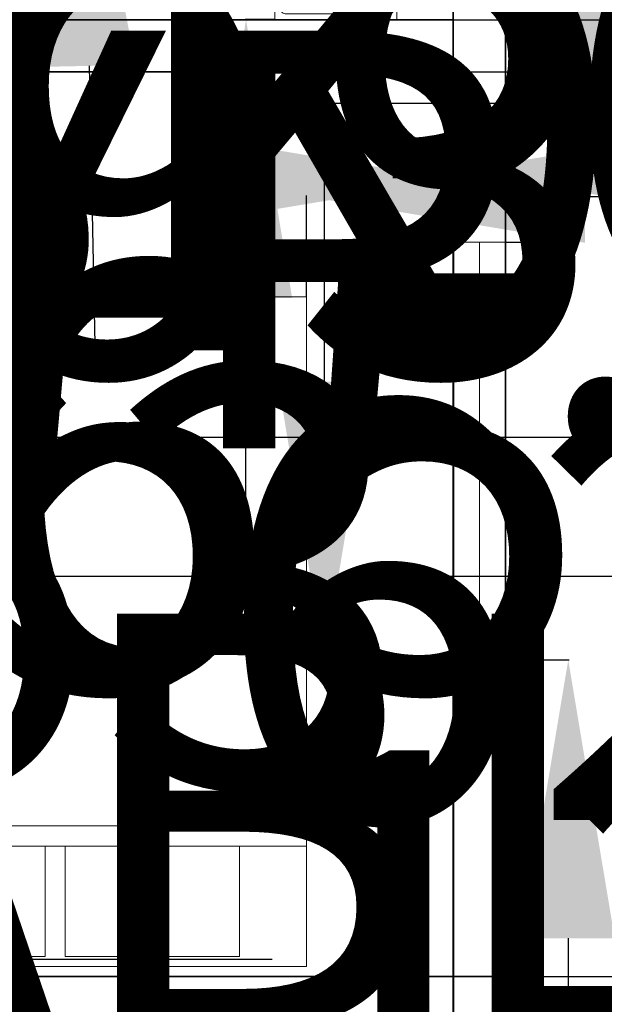
# Model space of a CAD drawing. Units: inches. Extents: x -307 to 2141, y -58 to 895.
# Tile 16 of 28: x 833 to 933, y 312 to 481. Entities that reach past the tile are written whole.
import ezdxf

# ---------------------------------------------------------------- set-up
doc = ezdxf.new("R2010")
doc.units = ezdxf.units.IN
doc.header["$MEASUREMENT"] = 0
for name, color, linetype, lineweight in [('A-ANNO-DIMS', 2, 'Continuous', 18), ('A-FLOR-FIXT', 9, 'Continuous', 18), ('A-FURN', 8, 'Continuous', 18), ('A-GLAZ', 4, 'Continuous', 18), ('A-WALL', 7, 'Continuous', 35)]:
    doc.layers.add(name, color=color, linetype=linetype, lineweight=lineweight)
doc.styles.get("Standard").update_dxf_attribs({"font": 'arial.ttf'})
doc.dimstyles.get("Standard").update_dxf_attribs({"dimtxt": 72, "dimasz": 48, "dimexe": 0.18, "dimexo": 0.0625, "dimgap": 0.09, "dimtad": 0, "dimtih": 1, "dimtoh": 1, "dimdec": 0, "dimrnd": 48, "dimzin": 0, "dimdsep": 46, "dimlunit": 3, "dimtxsty": 'Standard', "dimcen": 0.09, "dimadec": 0, "dimazin": 0, "dimtfac": 1, "dimtdec": 0, "dimtofl": 0, "dimtmove": 0, "dimatfit": 3, "dimfxl": 1, "dimtolj": 1, "dimtzin": 0, "dimarcsym": 0})

# ---------------------------------------------------------------- blocks, each defined once
blk = doc.blocks.new('Bed - Queen')
for p, q in [((0, -80.00003), (0, 0)), ((0, 0), (59.99999, 0)), ((59.99999, 0), (59.99999, -80.00003)), ((7.99999, -1.2), (28.79998, -1.2)), ((7.99999, -14.4), (7.99999, -1.2)), ((28.79998, -1.2), (28.79998, -14.4)), ((31.19999, -1.2), (51.99999, -1.2)), ((31.19999, -14.4), (31.19999, -1.2)), ((51.99999, -1.2), (51.99999, -16.4)), ((0, -14.4), (44.8, -14.4)), ((59.99999, -29.6), (44.8, -14.4)), ((44.8, -14.4), (44.8, -29.6)), ((51.99999, -16.4), (46.79936, -16.4)), ((44.8, -16.8), (0, -16.8)), ((44.8, -29.6), (59.99999, -29.6)), ((59.99999, -80.00003), (0, -80.00003))]:
    blk.add_line(p, q)
blk = doc.blocks.new('Toilet - top')
for p, q in [((9.5, -6), (9.5, -2)), ((-8, -8.5), (-8, -8)), ((-7, -8), (-7, -9.5)), ((-4, -8), (-6, -14)), ((4, -8), (6, -14)), ((-10, -8.5), (-8, -8.5)), ((-10, -9.5), (-10, -8.5)), ((-7, -9.5), (-10, -9.5)), ((4, -14), (-4, -14))]:
    blk.add_line(p, q)
blk.add_lwpolyline([(10.5, -8), (10.5, 0), (-10.5, 0), (-10.5, -8)], close=True)
for points in [[(8.5, -1), (-8.5, -1)], [(-9.5, -2), (-9.5, -6)], [(-8.5, -7), (8.5, -7)]]:
    blk.add_lwpolyline(points)
for centre, radius, start, end in [((-8.62, -1.88), 0.884, 81.8699, 188.1301), ((8.62, -1.88), 0.884, 351.8699, 98.1301), ((-8.62, -6.12), 0.884, 171.8699, 278.1301), ((8.62, -6.12), 0.884, 261.8699, 8.1301), ((3.52, -21.58), 12.17, 141.4691, 247.9714), ((4.2, -21.82), 11.33, 136.3677, 238.9468), ((-3.52, -21.58), 12.17, 292.0284, 38.5307), ((-4.2, -21.82), 11.33, 301.053, 43.6321), ((0, -27.88), 4, 245.7318, 294.2682), ((0, -29), 4, 254.8605, 285.1395)]:
    blk.add_arc(centre, radius, start, end)
blk = doc.blocks.new('WIN-36IN-PAIR')
for p, q in [((72.02, 9), (72.02, 0)), ((0, 4.5), (36, 4.5)), ((36.02, 4.5), (72.02, 4.5))]:
    blk.add_line(p, q)
for points in [[(36, 0), (0, 0), (0, 9), (36, 9)], [(36.02, 9), (72.02, 9)], [(72.02, 0), (36.02, 0)]]:
    blk.add_lwpolyline(points)
blk = doc.blocks.new('*D29')
at = {"layer": 'A-ANNO-DIMS', "color": 0, "lineweight": -2, "transparency": 16777216}
for p, q in [((747.42, 450.87), (699.42, 450.87)), ((795.42, 433.61), (795.42, 451.05)), ((882.03, 433.61), (882.03, 451.05)), ((930.03, 450.87), (978.03, 450.87))]:
    blk.add_line(p, q, dxfattribs=at)
at = {"layer": 'A-ANNO-DIMS', "color": 0, "transparency": 16777216}
for points in [[(747.42, 458.87), (747.42, 442.87), (795.42, 450.87)], [(930.03, 458.87), (930.03, 442.87), (882.03, 450.87)]]:
    blk.add_solid(points, dxfattribs=at)
at = {"layer": 'Defpoints', "color": 0, "transparency": 16777216}
for p in [(795.42, 450.87), (795.42, 433.55), (882.03, 433.55)]:
    blk.add_point(p, dxfattribs=at)
at = {"layer": 'A-ANNO-DIMS', "color": 0, "transparency": 16777216, "insert": (647.71, 450.87), "char_height": 72, "attachment_point": 5}
blk.add_mtext('\\A1;87', dxfattribs=at)
blk = doc.blocks.new('*D30')
at = {"layer": 'A-ANNO-DIMS', "color": 0, "lineweight": -2, "transparency": 16777216}
for p, q in [((570.74, 532.83), (570.74, 580.83)), ((570.74, 580.83), (618.74, 580.83)), ((565.4, 484.83), (570.92, 484.83)), ((565.4, 448.83), (570.92, 448.83)), ((570.74, 400.83), (570.74, 352.83))]:
    blk.add_line(p, q, dxfattribs=at)
at = {"layer": 'A-ANNO-DIMS', "color": 0, "transparency": 16777216}
for points in [[(562.74, 532.83), (578.74, 532.83), (570.74, 484.83)], [(562.74, 400.83), (578.74, 400.83), (570.74, 448.83)]]:
    blk.add_solid(points, dxfattribs=at)
at = {"layer": 'Defpoints', "color": 0, "transparency": 16777216}
for p in [(565.34, 484.83), (570.74, 484.83), (565.34, 448.83)]:
    blk.add_point(p, dxfattribs=at)
at = {"layer": 'A-ANNO-DIMS', "color": 0, "transparency": 16777216, "insert": (1030.17, 580.83), "char_height": 72, "attachment_point": 5}
blk.add_mtext('\\A1;WINDOW 36 TYP.', dxfattribs=at)
blk = doc.blocks.new('*D31')
at = {"layer": 'A-ANNO-DIMS', "color": 0, "lineweight": -2, "transparency": 16777216}
for p, q in [((556.34, 448.77), (556.34, 443.25)), ((565.34, 448.77), (565.34, 443.25)), ((508.34, 443.43), (460.34, 443.43)), ((613.34, 443.43), (661.34, 443.43))]:
    blk.add_line(p, q, dxfattribs=at)
at = {"layer": 'A-ANNO-DIMS', "color": 0, "transparency": 16777216}
for points in [[(508.34, 451.43), (508.34, 435.43), (556.34, 443.43)], [(613.34, 451.43), (613.34, 435.43), (565.34, 443.43)]]:
    blk.add_solid(points, dxfattribs=at)
at = {"layer": 'Defpoints', "color": 0, "transparency": 16777216}
for p in [(556.34, 448.83), (565.34, 448.83), (565.34, 443.43)]:
    blk.add_point(p, dxfattribs=at)
at = {"layer": 'A-ANNO-DIMS', "color": 0, "transparency": 16777216, "insert": (808.69, 443.43), "char_height": 72, "attachment_point": 5}
blk.add_mtext('\\A1;9 TYP.', dxfattribs=at)
blk = doc.blocks.new('*D34')
at = {"layer": 'A-ANNO-DIMS', "color": 0, "lineweight": -2, "transparency": 16777216}
for p, q in [((927.14, 490.97), (927.14, 538.97)), ((927.14, 538.97), (975.14, 538.97)), ((916.4, 442.97), (927.32, 442.97)), ((916.4, 370.95), (927.32, 370.95)), ((927.14, 322.95), (927.14, 274.95))]:
    blk.add_line(p, q, dxfattribs=at)
at = {"layer": 'A-ANNO-DIMS', "color": 0, "transparency": 16777216}
for points in [[(919.14, 490.97), (935.14, 490.97), (927.14, 442.97)], [(919.14, 322.95), (935.14, 322.95), (927.14, 370.95)]]:
    blk.add_solid(points, dxfattribs=at)
at = {"layer": 'Defpoints', "color": 0, "transparency": 16777216}
for p in [(916.34, 442.97), (927.14, 442.97), (916.34, 370.95)]:
    blk.add_point(p, dxfattribs=at)
at = {"layer": 'A-ANNO-DIMS', "color": 0, "transparency": 16777216, "insert": (1584.53, 538.97), "char_height": 72, "attachment_point": 5}
blk.add_mtext('\\A1;PAIRED WINDOW 72 TYP.', dxfattribs=at)
blk = doc.blocks.new('*D35')
at = {"layer": 'A-ANNO-DIMS', "color": 0, "lineweight": -2, "transparency": 16777216}
for p, q in [((859.34, 453.77), (811.34, 453.77)), ((907.34, 443.03), (907.34, 453.95)), ((916.34, 443.03), (916.34, 453.95)), ((964.34, 453.77), (1012.34, 453.77))]:
    blk.add_line(p, q, dxfattribs=at)
at = {"layer": 'A-ANNO-DIMS', "color": 0, "transparency": 16777216}
for points in [[(859.34, 461.77), (859.34, 445.77), (907.34, 453.77)], [(964.34, 461.77), (964.34, 445.77), (916.34, 453.77)]]:
    blk.add_solid(points, dxfattribs=at)
at = {"layer": 'Defpoints', "color": 0, "transparency": 16777216}
for p in [(907.34, 453.77), (907.34, 442.97), (916.34, 442.97)]:
    blk.add_point(p, dxfattribs=at)
at = {"layer": 'A-ANNO-DIMS', "color": 0, "transparency": 16777216, "insert": (663.98, 453.77), "char_height": 72, "attachment_point": 5}
blk.add_mtext('\\A1;9 TYP.', dxfattribs=at)
blk = doc.blocks.new('*D36')
at = {"layer": 'A-ANNO-DIMS', "color": 0, "lineweight": -2, "transparency": 16777216}
for p, q in [((871.71, 562.4), (871.76, 610.4)), ((876.55, 514.4), (871.47, 514.4)), ((876.51, 481.35), (871.44, 481.36)), ((871.56, 433.36), (871.51, 385.36)), ((871.51, 385.36), (823.51, 385.36))]:
    blk.add_line(p, q, dxfattribs=at)
at = {"layer": 'A-ANNO-DIMS', "color": 0, "transparency": 16777216}
for points in [[(863.71, 562.41), (879.71, 562.4), (871.65, 514.4)], [(863.56, 433.37), (879.56, 433.35), (871.62, 481.36)]]:
    blk.add_solid(points, dxfattribs=at)
at = {"layer": 'Defpoints', "color": 0, "transparency": 16777216}
for p in [(876.61, 514.4), (871.62, 481.36), (876.57, 481.35)]:
    blk.add_point(p, dxfattribs=at)
at = {"layer": 'A-ANNO-DIMS', "color": 0, "transparency": 16777216, "insert": (548.95, 385.36), "char_height": 72, "attachment_point": 5}
blk.add_mtext('\\A1;WC 33 TYP.', dxfattribs=at)
blk = doc.blocks.new('*D37')
at = {"layer": 'A-ANNO-DIMS', "color": 0, "lineweight": -2, "transparency": 16777216}
for p, q in [((876.61, 514.46), (876.62, 519.54)), ((828.62, 519.41), (780.62, 519.46)), ((897.61, 514.44), (897.62, 519.51)), ((945.62, 519.28), (993.62, 519.22))]:
    blk.add_line(p, q, dxfattribs=at)
at = {"layer": 'A-ANNO-DIMS', "color": 0, "transparency": 16777216}
for points in [[(828.63, 527.41), (828.61, 511.41), (876.62, 519.36)], [(945.63, 527.28), (945.61, 511.28), (897.62, 519.33)]]:
    blk.add_solid(points, dxfattribs=at)
at = {"layer": 'Defpoints', "color": 0, "transparency": 16777216}
for p in [(876.62, 519.36), (876.61, 514.4), (897.61, 514.38)]:
    blk.add_point(p, dxfattribs=at)
at = {"layer": 'A-ANNO-DIMS', "color": 0, "transparency": 16777216, "insert": (604.68, 519.46), "char_height": 72, "attachment_point": 5}
blk.add_mtext('\\A1;21 TYP.', dxfattribs=at)
blk = doc.blocks.new('*D41')
at = {"layer": 'A-ANNO-DIMS', "color": 0, "lineweight": -2, "transparency": 16777216}
for p, q in [((768.38, 207.13), (768.38, 255.13)), ((768.38, 255.13), (816.38, 255.13)), ((762.83, 159.13), (768.56, 159.13)), ((762.83, 128.96), (768.56, 128.96)), ((768.38, 80.96), (768.38, 32.96))]:
    blk.add_line(p, q, dxfattribs=at)
at = {"layer": 'A-ANNO-DIMS', "color": 0, "transparency": 16777216}
for points in [[(760.38, 207.13), (776.38, 207.13), (768.38, 159.13)], [(760.38, 80.96), (776.38, 80.96), (768.38, 128.96)]]:
    blk.add_solid(points, dxfattribs=at)
at = {"layer": 'Defpoints', "color": 0, "transparency": 16777216}
for p in [(762.77, 159.13), (768.38, 159.13), (762.77, 128.96)]:
    blk.add_point(p, dxfattribs=at)
at = {"layer": 'A-ANNO-DIMS', "color": 0, "transparency": 16777216, "insert": (991.68, 255.13), "char_height": 72, "attachment_point": 5}
blk.add_mtext('\\A1;30 TYP.', dxfattribs=at)
blk = doc.blocks.new('*D42')
at = {"layer": 'A-ANNO-DIMS', "color": 0, "lineweight": -2, "transparency": 16777216}
for p, q in [((880.26, 543.86), (928.25, 544.87)), ((774.28, 541.63), (726.29, 540.62)), ((822.3, 541.2), (822.27, 542.82)), ((832.3, 541.41), (832.27, 543.03))]:
    blk.add_line(p, q, dxfattribs=at)
at = {"layer": 'A-ANNO-DIMS', "color": 0, "transparency": 16777216}
for points in [[(880.09, 551.86), (880.43, 535.86), (832.27, 542.85)], [(774.11, 549.63), (774.45, 533.63), (822.27, 542.64)]]:
    blk.add_solid(points, dxfattribs=at)
at = {"layer": 'Defpoints', "color": 0, "transparency": 16777216}
for p in [(832.27, 542.85), (822.3, 541.14), (832.3, 541.35)]:
    blk.add_point(p, dxfattribs=at)
at = {"layer": 'A-ANNO-DIMS', "color": 0, "transparency": 16777216, "insert": (1192.89, 544.87), "char_height": 72, "attachment_point": 5}
blk.add_mtext('\\A1;FAUCET 10', dxfattribs=at)
blk = doc.blocks.new('*D44')
at = {"layer": 'A-ANNO-DIMS', "color": 0, "lineweight": -2, "transparency": 16777216}
for p, q in [((839.87, 521.22), (839.95, 517.42)), ((815.33, 520.71), (815.41, 516.91)), ((887.94, 518.61), (935.93, 519.62)), ((767.41, 516.08), (719.42, 515.07))]:
    blk.add_line(p, q, dxfattribs=at)
at = {"layer": 'A-ANNO-DIMS', "color": 0, "transparency": 16777216}
for points in [[(887.77, 526.61), (888.11, 510.61), (839.95, 517.6)], [(767.25, 524.08), (767.58, 508.08), (815.4, 517.09)]]:
    blk.add_solid(points, dxfattribs=at)
at = {"layer": 'Defpoints', "color": 0, "transparency": 16777216}
for p in [(839.87, 521.29), (815.33, 520.77), (839.95, 517.6)]:
    blk.add_point(p, dxfattribs=at)
at = {"layer": 'A-ANNO-DIMS', "color": 0, "transparency": 16777216, "insert": (1151.16, 519.62), "char_height": 72, "attachment_point": 5}
blk.add_mtext('\\A1;BASIN 25', dxfattribs=at)
blk = doc.blocks.new('*D45')
at = {"layer": 'A-ANNO-DIMS', "color": 0, "lineweight": -2, "transparency": 16777216}
for p, q in [((841.11, 637.47), (793.11, 637.47)), ((842.12, 589.48), (841.11, 637.47)), ((839.51, 541.42), (843.31, 541.5)), ((839.93, 521.29), (843.73, 521.37)), ((844.56, 473.37), (845.57, 425.38))]:
    blk.add_line(p, q, dxfattribs=at)
at = {"layer": 'A-ANNO-DIMS', "color": 0, "transparency": 16777216}
for points in [[(850.12, 589.65), (834.12, 589.32), (843.13, 541.49)], [(852.56, 473.54), (836.56, 473.21), (843.55, 521.36)]]:
    blk.add_solid(points, dxfattribs=at)
at = {"layer": 'Defpoints', "color": 0, "transparency": 16777216}
for p in [(839.45, 541.42), (843.13, 541.49), (839.87, 521.29)]:
    blk.add_point(p, dxfattribs=at)
at = {"layer": 'A-ANNO-DIMS', "color": 0, "transparency": 16777216, "insert": (740.96, 637.47), "char_height": 72, "attachment_point": 5}
blk.add_mtext('\\A1;20', dxfattribs=at)
blk = doc.blocks.new('*D46')
at = {"layer": 'A-ANNO-DIMS', "color": 0, "lineweight": -2, "transparency": 16777216}
for p, q in [((801.41, 645.78), (801.41, 642.52)), ((822.41, 645.78), (822.41, 642.52)), ((753.41, 642.7), (705.41, 642.7)), ((870.41, 642.7), (918.41, 642.7))]:
    blk.add_line(p, q, dxfattribs=at)
at = {"layer": 'A-ANNO-DIMS', "color": 0, "transparency": 16777216}
for points in [[(753.41, 650.7), (753.41, 634.7), (801.41, 642.7)], [(870.41, 650.7), (870.41, 634.7), (822.41, 642.7)]]:
    blk.add_solid(points, dxfattribs=at)
at = {"layer": 'Defpoints', "color": 0, "transparency": 16777216}
for p in [(801.41, 645.85), (822.41, 645.85), (822.41, 642.7)]:
    blk.add_point(p, dxfattribs=at)
at = {"layer": 'A-ANNO-DIMS', "color": 0, "transparency": 16777216, "insert": (1282.7, 642.7), "char_height": 72, "attachment_point": 5}
blk.add_mtext('\\A1;DESK CHAIR 21', dxfattribs=at)
blk = doc.blocks.new('*D52')
at = {"layer": 'A-ANNO-DIMS', "color": 0, "lineweight": -2, "transparency": 16777216}
for p, q in [((660.21, 554.25), (660.21, 602.25)), ((673.8, 506.25), (660.03, 506.25)), ((673.8, 415.25), (660.03, 415.25)), ((660.21, 367.25), (660.21, 319.25))]:
    blk.add_line(p, q, dxfattribs=at)
at = {"layer": 'A-ANNO-DIMS', "color": 0, "transparency": 16777216}
for points in [[(652.21, 554.25), (668.21, 554.25), (660.21, 506.25)], [(652.21, 367.25), (668.21, 367.25), (660.21, 415.25)]]:
    blk.add_solid(points, dxfattribs=at)
at = {"layer": 'Defpoints', "color": 0, "transparency": 16777216}
for p in [(673.86, 506.25), (660.21, 415.25), (673.86, 415.25)]:
    blk.add_point(p, dxfattribs=at)
at = {"layer": 'A-ANNO-DIMS', "color": 0, "transparency": 16777216, "insert": (660.21, 460.75), "char_height": 72, "attachment_point": 5}
blk.add_mtext('\\A1;DINING SET 91', dxfattribs=at)
blk = doc.blocks.new('*D53')
at = {"layer": 'A-ANNO-DIMS', "color": 0, "lineweight": -2, "transparency": 16777216}
for p, q in [((673.86, 415.19), (673.86, 401.42)), ((728.86, 415.19), (728.86, 401.42)), ((625.86, 401.6), (577.86, 401.6)), ((776.86, 401.6), (824.86, 401.6))]:
    blk.add_line(p, q, dxfattribs=at)
at = {"layer": 'A-ANNO-DIMS', "color": 0, "transparency": 16777216}
for points in [[(625.86, 409.6), (625.86, 393.6), (673.86, 401.6)], [(776.86, 409.6), (776.86, 393.6), (728.86, 401.6)]]:
    blk.add_solid(points, dxfattribs=at)
at = {"layer": 'Defpoints', "color": 0, "transparency": 16777216}
for p in [(673.86, 415.25), (728.86, 415.25), (728.86, 401.6)]:
    blk.add_point(p, dxfattribs=at)
at = {"layer": 'A-ANNO-DIMS', "color": 0, "transparency": 16777216, "insert": (876.79, 401.6), "char_height": 72, "attachment_point": 5}
blk.add_mtext('\\A1;55', dxfattribs=at)
blk = doc.blocks.new('*D54')
at = {"layer": 'A-ANNO-DIMS', "color": 0, "lineweight": -2, "transparency": 16777216}
for p, q in [((605.34, 412.35), (605.34, 460.35)), ((605.34, 460.35), (653.34, 460.35)), ((596.4, 364.35), (605.52, 364.35)), ((596.4, 304.35), (605.52, 304.35)), ((605.34, 256.35), (605.34, 208.35))]:
    blk.add_line(p, q, dxfattribs=at)
at = {"layer": 'A-ANNO-DIMS', "color": 0, "transparency": 16777216}
for points in [[(597.34, 412.35), (613.34, 412.35), (605.34, 364.35)], [(597.34, 256.35), (613.34, 256.35), (605.34, 304.35)]]:
    blk.add_solid(points, dxfattribs=at)
at = {"layer": 'Defpoints', "color": 0, "transparency": 16777216}
for p in [(596.34, 364.35), (605.34, 364.35), (596.34, 304.35)]:
    blk.add_point(p, dxfattribs=at)
at = {"layer": 'A-ANNO-DIMS', "color": 0, "transparency": 16777216, "insert": (854, 460.35), "char_height": 72, "attachment_point": 5}
blk.add_mtext('\\A1;DESK 60', dxfattribs=at)
blk = doc.blocks.new('*D60')
at = {"layer": 'A-ANNO-DIMS', "color": 0, "lineweight": -2, "transparency": 16777216}
for p, q in [((659.86, 294.95), (659.86, 342.95)), ((659.86, 342.95), (707.86, 342.95)), ((663.34, 246.95), (659.68, 246.95)), ((663.34, 223.32), (659.68, 223.32)), ((659.86, 175.32), (659.86, 127.32))]:
    blk.add_line(p, q, dxfattribs=at)
at = {"layer": 'A-ANNO-DIMS', "color": 0, "transparency": 16777216}
for points in [[(651.86, 294.95), (667.86, 294.95), (659.86, 246.95)], [(651.86, 175.32), (667.86, 175.32), (659.86, 223.32)]]:
    blk.add_solid(points, dxfattribs=at)
at = {"layer": 'Defpoints', "color": 0, "transparency": 16777216}
for p in [(659.86, 246.95), (663.4, 246.95), (663.4, 223.32)]:
    blk.add_point(p, dxfattribs=at)
at = {"layer": 'A-ANNO-DIMS', "color": 0, "transparency": 16777216, "insert": (933.57, 342.95), "char_height": 72, "attachment_point": 5}
blk.add_mtext('\\A1;TABLE 24', dxfattribs=at)
blk = doc.blocks.new('*D63')
at = {"layer": 'A-ANNO-DIMS', "color": 0, "lineweight": -2, "transparency": 16777216}
for p, q in [((916.4, 691.34), (947.72, 691.34)), ((947.54, 643.34), (947.54, 416.19)), ((947.54, 115.34), (947.54, 342.49)), ((704.68, 67.34), (947.72, 67.34))]:
    blk.add_line(p, q, dxfattribs=at)
at = {"layer": 'A-ANNO-DIMS', "color": 0, "transparency": 16777216}
for points in [[(939.54, 643.34), (955.54, 643.34), (947.54, 691.34)], [(939.54, 115.34), (955.54, 115.34), (947.54, 67.34)]]:
    blk.add_solid(points, dxfattribs=at)
at = {"layer": 'Defpoints', "color": 0, "transparency": 16777216}
for p in [(916.34, 691.34), (704.62, 67.34), (947.54, 67.34)]:
    blk.add_point(p, dxfattribs=at)
at = {"layer": 'A-ANNO-DIMS', "color": 0, "transparency": 16777216, "insert": (947.54, 379.34), "char_height": 72, "attachment_point": 5}
blk.add_mtext('\\A1;624', dxfattribs=at)
blk = doc.blocks.new('*D81')
at = {"layer": 'A-ANNO-DIMS', "color": 0, "lineweight": -2, "transparency": 16777216}
for p, q in [((947.54, 589.34), (947.54, 637.34)), ((947.54, 637.34), (995.54, 637.34)), ((907.4, 541.34), (947.72, 541.34)), ((907.4, 481.34), (947.72, 481.34)), ((947.54, 433.34), (947.54, 385.34))]:
    blk.add_line(p, q, dxfattribs=at)
at = {"layer": 'A-ANNO-DIMS', "color": 0, "transparency": 16777216}
for points in [[(939.54, 589.34), (955.54, 589.34), (947.54, 541.34)], [(939.54, 433.34), (955.54, 433.34), (947.54, 481.34)]]:
    blk.add_solid(points, dxfattribs=at)
at = {"layer": 'Defpoints', "color": 0, "transparency": 16777216}
for p in [(907.34, 541.34), (947.54, 541.34), (907.34, 481.34)]:
    blk.add_point(p, dxfattribs=at)
at = {"layer": 'A-ANNO-DIMS', "color": 0, "transparency": 16777216, "insert": (1047.27, 637.34), "char_height": 72, "attachment_point": 5}
blk.add_mtext('\\A1;60', dxfattribs=at)
blk = doc.blocks.new('*D83')
at = {"layer": 'A-ANNO-DIMS', "color": 0, "lineweight": -2, "transparency": 16777216}
for p, q in [((947.54, 538.9), (947.54, 586.9)), ((916.4, 490.9), (947.72, 490.9)), ((907.4, 481.34), (947.72, 481.34)), ((947.54, 433.34), (947.54, 385.34)), ((947.54, 385.34), (899.54, 385.34))]:
    blk.add_line(p, q, dxfattribs=at)
at = {"layer": 'A-ANNO-DIMS', "color": 0, "transparency": 16777216}
for points in [[(939.54, 538.9), (955.54, 538.9), (947.54, 490.9)], [(939.54, 433.34), (955.54, 433.34), (947.54, 481.34)]]:
    blk.add_solid(points, dxfattribs=at)
at = {"layer": 'Defpoints', "color": 0, "transparency": 16777216}
for p in [(916.34, 490.9), (907.34, 481.34), (947.54, 481.34)]:
    blk.add_point(p, dxfattribs=at)
at = {"layer": 'A-ANNO-DIMS', "color": 0, "transparency": 16777216, "insert": (777.97, 385.34), "char_height": 72, "attachment_point": 5}
blk.add_mtext('\\A1;9.563', dxfattribs=at)
blk = doc.blocks.new('*D84')
at = {"layer": 'A-ANNO-DIMS', "color": 0, "lineweight": -2, "transparency": 16777216}
for p, q in [((763.34, 472.28), (763.34, 35.96)), ((907.34, 472.28), (907.34, 35.96)), ((811.34, 36.14), (859.34, 36.14)), ((907.34, 36.14), (955.34, 36.14))]:
    blk.add_line(p, q, dxfattribs=at)
at = {"layer": 'A-ANNO-DIMS', "color": 0, "transparency": 16777216}
for points in [[(811.34, 44.14), (811.34, 28.14), (763.34, 36.14)], [(859.34, 44.14), (859.34, 28.14), (907.34, 36.14)]]:
    blk.add_solid(points, dxfattribs=at)
at = {"layer": 'Defpoints', "color": 0, "transparency": 16777216}
for p in [(763.34, 472.34), (907.34, 472.34), (907.34, 36.14)]:
    blk.add_point(p, dxfattribs=at)
at = {"layer": 'A-ANNO-DIMS', "color": 0, "transparency": 16777216, "insert": (1031.43, 36.14), "char_height": 72, "attachment_point": 5}
blk.add_mtext('\\A1;144', dxfattribs=at)
blk = doc.blocks.new('*D85')
at = {"layer": 'A-ANNO-DIMS', "color": 0, "lineweight": -2, "transparency": 16777216}
for p, q in [((947.54, 472.34), (947.54, 520.34)), ((947.54, 520.34), (995.54, 520.34)), ((907.4, 472.34), (947.72, 472.34)), ((947.54, 364.34), (947.54, 424.34)), ((916.4, 316.34), (947.72, 316.34))]:
    blk.add_line(p, q, dxfattribs=at)
at = {"layer": 'A-ANNO-DIMS', "color": 0, "transparency": 16777216}
for points in [[(939.54, 424.34), (955.54, 424.34), (947.54, 472.34)], [(939.54, 364.34), (955.54, 364.34), (947.54, 316.34)]]:
    blk.add_solid(points, dxfattribs=at)
at = {"layer": 'Defpoints', "color": 0, "transparency": 16777216}
for p in [(907.34, 472.34), (947.54, 472.34), (916.34, 316.34)]:
    blk.add_point(p, dxfattribs=at)
at = {"layer": 'A-ANNO-DIMS', "color": 0, "transparency": 16777216, "insert": (1071.76, 520.34), "char_height": 72, "attachment_point": 5}
blk.add_mtext('\\A1;156', dxfattribs=at)
blk = doc.blocks.new('*D88')
at = {"layer": 'A-ANNO-DIMS', "color": 0, "lineweight": -2, "transparency": 16777216}
for p, q in [((517.33584, 722.544828), (469.33584, 722.544828)), ((565.33584, 295.403328), (565.33584, 722.724828)), ((754.33584, 271.403328), (754.33584, 722.724828)), ((802.33584, 722.544828), (850.33584, 722.544828))]:
    blk.add_line(p, q, dxfattribs=at)
at = {"layer": 'A-ANNO-DIMS', "color": 0, "transparency": 16777216}
for points in [[(517.33584, 730.544828), (517.33584, 714.544828), (565.33584, 722.544828)], [(802.33584, 730.544828), (802.33584, 714.544828), (754.33584, 722.544828)]]:
    blk.add_solid(points, dxfattribs=at)
at = {"layer": 'Defpoints', "color": 0, "transparency": 16777216}
for p in [(754.33584, 722.544828), (565.33584, 295.340828), (754.33584, 271.340828)]:
    blk.add_point(p, dxfattribs=at)
at = {"layer": 'A-ANNO-DIMS', "color": 0, "transparency": 16777216, "insert": (659.83584, 722.544828), "char_height": 72, "attachment_point": 5}
blk.add_mtext('\\A1;189', dxfattribs=at)
blk = doc.blocks.new('*D95')
at = {"layer": 'A-ANNO-DIMS', "color": 0, "lineweight": -2, "transparency": 16777216}
for p, q in [((947.54, 577.34), (947.54, 625.34)), ((947.54, 625.34), (995.54, 625.34)), ((629.9, 529.34), (947.72, 529.34)), ((629.9, 502.66), (947.72, 502.66)), ((947.54, 454.66), (947.54, 406.66))]:
    blk.add_line(p, q, dxfattribs=at)
at = {"layer": 'A-ANNO-DIMS', "color": 0, "transparency": 16777216}
for points in [[(939.54, 577.34), (955.54, 577.34), (947.54, 529.34)], [(939.54, 454.66), (955.54, 454.66), (947.54, 502.66)]]:
    blk.add_solid(points, dxfattribs=at)
at = {"layer": 'Defpoints', "color": 0, "transparency": 16777216}
for p in [(629.84, 529.34), (947.54, 529.34), (629.84, 502.66)]:
    blk.add_point(p, dxfattribs=at)
at = {"layer": 'A-ANNO-DIMS', "color": 0, "transparency": 16777216, "insert": (1117.8, 625.34), "char_height": 72, "attachment_point": 5}
blk.add_mtext('\\A1;26.68', dxfattribs=at)
blk = doc.blocks.new('*D97')
at = {"layer": 'A-ANNO-DIMS', "color": 0, "lineweight": -2, "transparency": 16777216}
for p, q in [((947.54, 637.34), (947.54, 685.34)), ((947.54, 685.34), (995.54, 685.34)), ((685.4, 589.34), (947.72, 589.34)), ((685.4, 538.34), (947.72, 538.34)), ((947.54, 490.34), (947.54, 442.34))]:
    blk.add_line(p, q, dxfattribs=at)
at = {"layer": 'A-ANNO-DIMS', "color": 0, "transparency": 16777216}
for points in [[(939.54, 637.34), (955.54, 637.34), (947.54, 589.34)], [(939.54, 490.34), (955.54, 490.34), (947.54, 538.34)]]:
    blk.add_solid(points, dxfattribs=at)
at = {"layer": 'Defpoints', "color": 0, "transparency": 16777216}
for p in [(685.34, 589.34), (947.54, 589.34), (685.34, 538.34)]:
    blk.add_point(p, dxfattribs=at)
at = {"layer": 'A-ANNO-DIMS', "color": 0, "transparency": 16777216, "insert": (1040.25, 685.34), "char_height": 72, "attachment_point": 5}
blk.add_mtext('\\A1;51', dxfattribs=at)
blk = doc.blocks.new('*D99')
at = {"layer": 'A-ANNO-DIMS', "color": 0, "lineweight": -2, "transparency": 16777216}
for p, q in [((763.34, 481.28), (763.34, 35.96)), ((802.34, 481.28), (802.34, 35.96)), ((715.34, 36.14), (667.34, 36.14)), ((850.34, 36.14), (898.34, 36.14))]:
    blk.add_line(p, q, dxfattribs=at)
at = {"layer": 'A-ANNO-DIMS', "color": 0, "transparency": 16777216}
for points in [[(715.34, 44.14), (715.34, 28.14), (763.34, 36.14)], [(850.34, 44.14), (850.34, 28.14), (802.34, 36.14)]]:
    blk.add_solid(points, dxfattribs=at)
at = {"layer": 'Defpoints', "color": 0, "transparency": 16777216}
for p in [(763.34, 481.34), (802.34, 481.34), (802.34, 36.14)]:
    blk.add_point(p, dxfattribs=at)
at = {"layer": 'A-ANNO-DIMS', "color": 0, "transparency": 16777216, "insert": (950.04, 36.14), "char_height": 72, "attachment_point": 5}
blk.add_mtext('\\A1;39', dxfattribs=at)
blk = doc.blocks.new('*D104')
at = {"layer": 'A-ANNO-DIMS', "color": 0, "lineweight": -2, "transparency": 16777216}
for p, q in [((885.13, 418.95), (885.13, 466.95)), ((885.13, 466.95), (933.13, 466.95)), ((916.27, 370.95), (884.95, 370.95)), ((916.27, 307.34), (884.95, 307.34)), ((885.13, 259.34), (885.13, 211.34))]:
    blk.add_line(p, q, dxfattribs=at)
at = {"layer": 'A-ANNO-DIMS', "color": 0, "transparency": 16777216}
for points in [[(877.13, 418.95), (893.13, 418.95), (885.13, 370.95)], [(877.13, 259.34), (893.13, 259.34), (885.13, 307.34)]]:
    blk.add_solid(points, dxfattribs=at)
at = {"layer": 'Defpoints', "color": 0, "transparency": 16777216}
for p in [(885.13, 370.95), (916.34, 370.95), (916.34, 307.34)]:
    blk.add_point(p, dxfattribs=at)
at = {"layer": 'A-ANNO-DIMS', "color": 0, "transparency": 16777216, "insert": (1047.95, 466.95), "char_height": 72, "attachment_point": 5}
blk.add_mtext('\\A1;63.61', dxfattribs=at)
blk = doc.blocks.new('*D105')
at = {"layer": 'A-ANNO-DIMS', "color": 0, "lineweight": -2, "transparency": 16777216}
for p, q in [((828.13, 271.34), (828.13, 319.34)), ((828.13, 319.34), (876.13, 319.34)), ((859.27, 223.34), (827.95, 223.34)), ((859.27, 211.34), (827.95, 211.34)), ((828.13, 163.34), (828.13, 115.34))]:
    blk.add_line(p, q, dxfattribs=at)
at = {"layer": 'A-ANNO-DIMS', "color": 0, "transparency": 16777216}
for points in [[(820.13, 271.34), (836.13, 271.34), (828.13, 223.34)], [(820.13, 163.34), (836.13, 163.34), (828.13, 211.34)]]:
    blk.add_solid(points, dxfattribs=at)
at = {"layer": 'Defpoints', "color": 0, "transparency": 16777216}
for p in [(828.13, 223.34), (859.34, 223.34), (859.34, 211.34)]:
    blk.add_point(p, dxfattribs=at)
at = {"layer": 'A-ANNO-DIMS', "color": 0, "transparency": 16777216, "insert": (924.03, 319.34), "char_height": 72, "attachment_point": 5}
blk.add_mtext('\\A1;12', dxfattribs=at)
blk = doc.blocks.new('*D107')
at = {"layer": 'A-ANNO-DIMS', "color": 0, "lineweight": -2, "transparency": 16777216}
for p, q in [((517.34, 722.54), (469.34, 722.54)), ((565.34, 409.4), (565.34, 722.72)), ((589.34, 409.4), (589.34, 722.72)), ((637.34, 722.54), (685.34, 722.54))]:
    blk.add_line(p, q, dxfattribs=at)
at = {"layer": 'A-ANNO-DIMS', "color": 0, "transparency": 16777216}
for points in [[(517.34, 730.54), (517.34, 714.54), (565.34, 722.54)], [(637.34, 730.54), (637.34, 714.54), (589.34, 722.54)]]:
    blk.add_solid(points, dxfattribs=at)
at = {"layer": 'Defpoints', "color": 0, "transparency": 16777216}
for p in [(589.34, 722.54), (565.34, 409.34), (589.34, 409.34)]:
    blk.add_point(p, dxfattribs=at)
at = {"layer": 'A-ANNO-DIMS', "color": 0, "transparency": 16777216, "insert": (835.49, 722.54), "char_height": 72, "attachment_point": 5}
blk.add_mtext('\\A1;24.003', dxfattribs=at)
blk = doc.blocks.new('*D108')
at = {"layer": 'A-ANNO-DIMS', "color": 0, "lineweight": -2, "transparency": 16777216}
for p, q in [((947.54, 550.66), (947.54, 598.66)), ((589.4, 502.66), (947.72, 502.66)), ((589.4, 409.34), (947.72, 409.34)), ((947.54, 361.34), (947.54, 313.34))]:
    blk.add_line(p, q, dxfattribs=at)
at = {"layer": 'A-ANNO-DIMS', "color": 0, "transparency": 16777216}
for points in [[(939.54, 550.66), (955.54, 550.66), (947.54, 502.66)], [(939.54, 361.34), (955.54, 361.34), (947.54, 409.34)]]:
    blk.add_solid(points, dxfattribs=at)
at = {"layer": 'Defpoints', "color": 0, "transparency": 16777216}
for p in [(589.34, 502.66), (947.54, 502.66), (589.34, 409.34)]:
    blk.add_point(p, dxfattribs=at)
at = {"layer": 'A-ANNO-DIMS', "color": 0, "transparency": 16777216, "insert": (947.54, 456), "char_height": 72, "attachment_point": 5}
blk.add_mtext('\\A1;93.32', dxfattribs=at)
blk = doc.blocks.new('*D109')
at = {"layer": 'A-ANNO-DIMS', "color": 0, "lineweight": -2, "transparency": 16777216}
for p, q in [((723.13, 355.34), (723.13, 403.34)), ((723.13, 403.34), (771.13, 403.34)), ((754.27, 307.34), (722.95, 307.34)), ((754.27, 271.34), (722.95, 271.34)), ((723.13, 223.34), (723.13, 175.34))]:
    blk.add_line(p, q, dxfattribs=at)
at = {"layer": 'A-ANNO-DIMS', "color": 0, "transparency": 16777216}
for points in [[(715.13, 355.34), (731.13, 355.34), (723.13, 307.34)], [(715.13, 223.34), (731.13, 223.34), (723.13, 271.34)]]:
    blk.add_solid(points, dxfattribs=at)
at = {"layer": 'Defpoints', "color": 0, "transparency": 16777216}
for p in [(723.13, 307.34), (754.34, 307.34), (754.34, 271.34)]:
    blk.add_point(p, dxfattribs=at)
at = {"layer": 'A-ANNO-DIMS', "color": 0, "transparency": 16777216, "insert": (822.74, 403.34), "char_height": 72, "attachment_point": 5}
blk.add_mtext('\\A1;36', dxfattribs=at)

msp = doc.modelspace()

# ---------------------------------------------------------------- linework, layer by layer
at = {"layer": 'A-WALL'}
for p, q in [((916.3358, 166.3408), (916.3358, 691.3408)), ((907.3358, 166.3408), (907.3358, 682.3408)), ((907.3358, 481.3408), (802.3358, 481.3408)), ((907.3358, 481.3408), (802.3358, 481.3408)), ((907.3358, 472.3408), (802.3358, 472.3408)), ((916.3358, 316.3408), (754.3358, 316.3408))]:
    msp.add_line(p, q, dxfattribs=at)

# ---------------------------------------------------------------- block references
at = {"layer": 'A-FLOR-FIXT', "rotation": 179.9358923931402}
msp.add_blockref('Toilet - top', (887.0736, 481.3408), dxfattribs=at)
at = {"layer": 'A-FURN', "xscale": 1.443457686913744, "yscale": 1.443457686913744, "zscale": 1.443457686913744, "rotation": 179.9999999999998}
msp.add_blockref('Bed - Queen', (882.0282, 318.073), dxfattribs=at)
at = {"layer": 'A-GLAZ', "rotation": 89.99999999999979}
msp.add_blockref('WIN-36IN-PAIR', (916.3357, 370.9518), dxfattribs=at)

# ---------------------------------------------------------------- dimensions: what is measured, and where the dimension line sits
at = {"layer": 'A-ANNO-DIMS'}
for base, p1, p2, text, picture, middle in [((822.4132, 642.696), (801.4132, 645.846), (822.4132, 645.846), 'DESK CHAIR <>', '*D46', (1282.7024, 642.696)), ((565.3358, 443.4333), (556.3358, 448.8333), (565.3358, 448.8333), '<> TYP.', '*D31', (808.6919, 443.4333))]:
    dim = msp.add_linear_dim(base=base, p1=p1, p2=p2, text=text, dimstyle='Standard', override={"dimdec": 0, "dimlfac": 1, "dimrnd": 0, "dimzin": 0, "dimdsep": 46, "dimlunit": 2}, dxfattribs=at)
    dim.commit()
    dim.dimension.update_dxf_attribs({"geometry": picture, "text_midpoint": middle})
for base, p1, p2, override, picture, middle in [((754.3358, 722.5448), (565.3358, 295.3408), (754.3358, 271.3408), {"dimdec": 0, "dimlfac": 1, "dimrnd": 0, "dimzin": 0, "dimdsep": 46, "dimlunit": 2}, '*D88', (659.8358, 722.5448)), ((589.339, 722.5448), (565.3358, 409.3408), (589.339, 409.3408), {"dimdec": 3, "dimlfac": 1, "dimrnd": 0, "dimzin": 0, "dimdsep": 46, "dimlunit": 2}, '*D107', (835.4945, 722.5448)), ((802.3358, 36.1368), (763.3358, 481.3408), (802.3358, 481.3408), {"dimdec": 0, "dimlfac": 1, "dimrnd": 0, "dimzin": 0, "dimdsep": 46, "dimlunit": 2}, '*D99', (950.0438, 36.1368)), ((907.3358, 36.1368), (763.3358, 472.3408), (907.3358, 472.3408), {"dimdec": 0, "dimlfac": 1, "dimrnd": 0, "dimzin": 0, "dimdsep": 46, "dimlunit": 2}, '*D84', (1031.4286, 36.1368)), ((728.8583, 401.5985), (673.8583, 415.2485), (728.8583, 415.2485), {"dimdec": 0, "dimlfac": 1, "dimrnd": 0, "dimzin": 0, "dimdsep": 46, "dimlunit": 2}, '*D53', (876.7874, 401.5985))]:
    dim = msp.add_linear_dim(base=base, p1=p1, p2=p2, dimstyle='Standard', override=override, dxfattribs=at)
    dim.commit()
    dim.dimension.update_dxf_attribs({"geometry": picture, "text_midpoint": middle})
for base, p1, p2, angle, text, picture, middle in [((927.1381, 442.9669), (916.3358, 370.9517), (916.3358, 442.9669), 90, 'PAIRED WINDOW <> TYP.', '*D34', (1584.5269, 538.9669)), ((570.7358, 484.8333), (565.3358, 448.8333), (565.3358, 484.8333), 90, 'WINDOW <> TYP.', '*D30', (1030.1737, 580.8333)), ((832.2692, 542.8502), (822.3029, 541.1403), (832.3007, 541.3505), 1.204628, 'FAUCET <>', '*D42', (1192.8864, 544.8684)), ((660.2083, 415.2485), (673.8583, 506.2485), (673.8583, 415.2485), 270, 'DINING SET <>', '*D52', (660.2083, 460.7485)), ((876.6162, 519.3557), (897.6106, 514.3753), (876.6106, 514.3988), 179.935892, '<> TYP.', '*D37', (604.6763, 519.4631)), ((839.9481, 517.6035), (815.3253, 520.7692), (839.8707, 521.2853), 1.204628, 'BASIN <>', '*D44', (1151.1574, 519.6217)), ((871.6167, 481.3581), (876.6106, 514.3988), (876.5736, 481.3526), 269.935892, 'WC <> TYP.', '*D36', (548.95, 385.3582)), ((605.3358, 364.3488), (596.3358, 304.3488), (596.3358, 364.3488), 90, 'DESK <>', '*D54', (854.0043, 460.3488)), ((907.3358, 453.7692), (916.3358, 442.9669), (907.3358, 442.9669), 180, '<> TYP.', '*D35', (663.9798, 453.7692)), ((659.8571, 246.9465), (663.4018, 223.3153), (663.4018, 246.9465), 90, 'TABLE <>', '*D60', (933.5733, 342.9465)), ((768.3792, 159.1282), (762.7703, 128.9569), (762.7703, 159.1282), 90, '<> TYP.', '*D41', (991.6806, 255.1282))]:
    dim = msp.add_linear_dim(base=base, p1=p1, p2=p2, angle=angle, text=text, dimstyle='Standard', override={"dimdec": 0, "dimlfac": 1, "dimrnd": 0, "dimzin": 0, "dimdsep": 46, "dimlunit": 2}, dxfattribs=at)
    dim.commit()
    dim.dimension.update_dxf_attribs({"geometry": picture, "text_midpoint": middle})
for base, p1, p2, angle, override, picture, middle in [((947.5398, 589.3408), (685.3358, 538.3408), (685.3358, 589.3408), 90, {"dimdec": 0, "dimlfac": 1, "dimrnd": 0, "dimzin": 0, "dimdsep": 46, "dimlunit": 2}, '*D97', (1040.2492, 685.3408)), ((947.5398, 67.3408), (916.3358, 691.3408), (704.6211, 67.3408), 90, {"dimdec": 0, "dimlfac": 1, "dimrnd": 0, "dimzin": 0, "dimdsep": 46, "dimlunit": 2}, '*D63', (947.5398, 379.3408)), ((843.1292, 541.4949), (839.8707, 521.2853), (839.4474, 541.4175), 91.204628, {"dimdec": 0, "dimlfac": 1, "dimrnd": 0, "dimzin": 0, "dimdsep": 46, "dimlunit": 2}, '*D45', (740.961, 637.4737)), ((947.5398, 541.3408), (907.3358, 481.3408), (907.3358, 541.3408), 90, {"dimdec": 0, "dimlfac": 1, "dimrnd": 0, "dimzin": 0, "dimdsep": 46, "dimlunit": 2}, '*D81', (1047.2724, 637.3408)), ((947.5398, 529.3408), (629.8358, 502.6632), (629.8358, 529.3408), 90, {"dimdec": 2, "dimlfac": 1, "dimrnd": 0, "dimzin": 0, "dimdsep": 46, "dimlunit": 2}, '*D95', (1117.799, 625.3408)), ((947.5398, 502.6632), (589.339, 409.3408), (589.339, 502.6632), 90, {"dimdec": 2, "dimlfac": 1, "dimrnd": 0, "dimzin": 0, "dimdsep": 46, "dimlunit": 2}, '*D108', (947.5398, 456.002)), ((947.5398, 481.3408), (916.3358, 490.9034), (907.3358, 481.3408), 90, {"dimdec": 3, "dimlfac": 1, "dimrnd": 0, "dimzin": 0, "dimdsep": 46, "dimlunit": 2}, '*D83', (777.9683, 385.3408)), ((947.5398, 472.3408), (916.3358, 316.3408), (907.3358, 472.3408), 90, {"dimdec": 0, "dimlfac": 1, "dimrnd": 0, "dimzin": 0, "dimdsep": 46, "dimlunit": 2}, '*D85', (1071.7554, 520.3408)), ((885.1318, 370.9517), (916.3358, 307.3408), (916.3358, 370.9517), 90, {"dimdec": 2, "dimlfac": 1, "dimrnd": 0, "dimzin": 0, "dimdsep": 46, "dimlunit": 2}, '*D104', (1047.9504, 466.9517)), ((795.4208, 450.8711), (882.0282, 433.5496), (795.4208, 433.5496), 180, {"dimdec": 0, "dimlfac": 1, "dimrnd": 0, "dimzin": 0, "dimdsep": 46, "dimlunit": 2}, '*D29', (647.7128, 450.8711)), ((723.1318, 307.3408), (754.3358, 271.3408), (754.3358, 307.3408), 90, {"dimdec": 0, "dimlfac": 1, "dimrnd": 0, "dimzin": 0, "dimdsep": 46, "dimlunit": 2}, '*D109', (822.7416, 403.3408)), ((828.1318, 223.3408), (859.3358, 211.3408), (859.3358, 223.3408), 90, {"dimdec": 0, "dimlfac": 1, "dimrnd": 0, "dimzin": 0, "dimdsep": 46, "dimlunit": 2}, '*D105', (924.0336, 319.3408))]:
    dim = msp.add_linear_dim(base=base, p1=p1, p2=p2, angle=angle, dimstyle='Standard', override=override, dxfattribs=at)
    dim.commit()
    dim.dimension.update_dxf_attribs({"geometry": picture, "text_midpoint": middle})

doc.saveas('drawing.dxf')
